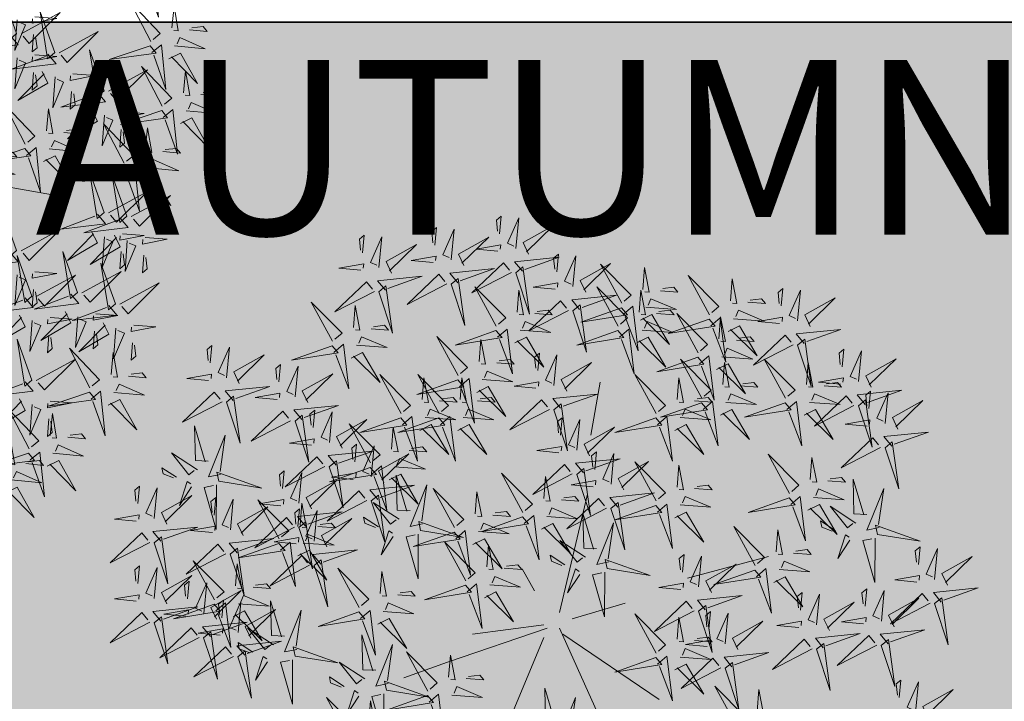
# Model space of a CAD drawing. Units: inches. Extents: x 1704 to 6393, y -157 to 1172.
# Tile 71 of 122: x 1920 to 1954, y 1010 to 1033. Entities that reach past the tile are written whole.
import ezdxf

# ---------------------------------------------------------------- set-up
doc = ezdxf.new("R2010")
doc.units = ezdxf.units.IN
doc.header["$MEASUREMENT"] = 0
for name, color, linetype, lineweight in [('A-ANNO-DIMS', 7, 'Continuous', 13), ('C-PROP', 7, 'Continuous', 35), ('L-shrub', 74, 'Continuous', 18), ('L-tree', 102, 'Continuous', 18)]:
    doc.layers.add(name, color=color, linetype=linetype, lineweight=lineweight)
doc.layers.add('L-HRDS-PATT', color=9, linetype='Continuous', lineweight=13, true_color=0xc5c1ba)
doc.styles.get("Standard").update_dxf_attribs({"font": 'arial.ttf'})
doc.dimstyles.get("Standard").update_dxf_attribs({"dimtxt": 6, "dimasz": 2, "dimexe": 0.18, "dimexo": 0.0625, "dimgap": 0.09, "dimtad": 0, "dimtih": 1, "dimtoh": 1, "dimdec": 1, "dimzin": 0, "dimdsep": 46, "dimlunit": 3, "dimtxsty": 'Standard', "dimblk": 'ARCHTICK', "dimcen": 0.09, "dimadec": 0, "dimazin": 0, "dimtfac": 1, "dimtdec": 1, "dimtofl": 0, "dimtmove": 0, "dimatfit": 3, "dimfxl": 1, "dimtolj": 1, "dimtzin": 0, "dimarcsym": 0})

# ---------------------------------------------------------------- blocks, each defined once
blk = doc.blocks.new('bamboo')
blk.add_line((390, 162.3), (546.4, 218.1))
at = {"layer": 'L-shrub'}
for p, q in [((43.5, 73), (278.2, 631.2)), ((-12.4, 39.5), (-247.1, 564.2)), ((-23.6, 61.9), (-370, 296.3)), ((32.3, 39.5), (390, 162.3)), ((43.5, 28.4), (300.5, 61.9)), ((-57.1, 6), (-247.1, -49.8)), ((-12.4, -16.3), (-113, -440.5)), ((77, -94.4), (121.7, -172.6)), ((-470.6, -139.1), (-761.2, -217.2)), ((-124.2, -652.6), (-157.7, -842.3))]:
    blk.add_line(p, q, dxfattribs=at)
for points in [[(-52.8, 429.4), (-9, 438.6), (-69, 289.1), (-50.5, 418.5)], [(455.6, 305.5), (421.7, 276.4), (402.2, 436.3), (448.3, 314)], [(617.5, 275.9), (618.2, 435.7), (661.3, 285.1), (628.5, 278.2)], [(747.2, 429.2), (823.6, 288.8), (713.3, 400), (738.7, 421.9)], [(672.1, 379.4), (666.1, 300.6), (649, 389), (664.8, 387.8)], [(-1334.9, 362.3), (-1315.1, 320.7), (-1424, 259.8), (-1327.8, 353.7)], [(-645.4, 388.3), (-569, 247.9), (-679.3, 359.1), (-653.9, 381)], [(-8.5, 381.7), (37.5, 380), (40.9, 255.2), (2.4, 384)], [(-1289.2, 342), (-1299.8, 231.9), (-1259.3, 323.3), (-1282.1, 333.4)], [(-720.5, 338.5), (-726.5, 259.7), (-743.5, 348.1), (-727.8, 346.9)], [(-606.2, 183.8), (-655.6, 331.4), (-632, 162.5), (-606.2, 183.8)], [(461.7, 281.3), (608.2, 333.7), (439.8, 306.7), (461.7, 281.3)], [(707.3, 283.4), (750.5, 349.5), (722.8, 263.8), (709.6, 272.4)], [(-1230.9, 288.8), (-1236.9, 225.9), (-1219.6, 240.1), (-1223.8, 280.1)], [(-363.6, 169.2), (-397.5, 140), (-417, 299.9), (-370.9, 177.6)], [(374.4, 279.9), (264.1, 288.2), (356.3, 249.6), (365.9, 272.6)], [(608.9, 262.7), (455.2, 287.4), (615.8, 229.9), (608.9, 262.7)], [(945.2, 153.2), (945.8, 313), (988.9, 162.4), (956.1, 155.5)], [(1141.3, 142.9), (1092, 290.5), (1115.5, 121.6), (1141.3, 142.9)], [(-1166, 102), (-1215.3, 249.6), (-1191.8, 80.7), (-1166, 102)], [(-933.9, 115.6), (-983.2, 263.3), (-959.7, 94.3), (-933.9, 115.6)], [(-590.5, 182.3), (-448.6, 255.9), (-562, 147.8), (-583.4, 173.7)], [(-425.4, 189.6), (-466.6, 169), (-529.7, 276.7), (-433.9, 182.4)], [(460.4, 265.6), (536.9, 125.2), (426.5, 236.4), (452, 258.3)], [(602.5, 238.5), (646.3, 247.7), (586.3, 98.2), (604.8, 227.6)], [(760.2, 248.9), (813.2, 214.4), (808.6, 236.2), (771.2, 251.2)], [(322.4, 220.5), (259.3, 225.2), (273.9, 208.3), (313.9, 213.2)], [(385.4, 215.7), (379.4, 137), (362.3, 225.4), (378.1, 224.2)], [(686, 221.8), (778.6, 161.5), (716.5, 239.7), (696.9, 224.1)], [(1035, 160.6), (1078.2, 226.8), (1050.5, 141.1), (1037.3, 149.7)], [(1157.1, 141.4), (1299, 214.9), (1185.5, 106.9), (1164.2, 132.8)], [(1264.2, 74.7), (1214.8, 222.3), (1238.4, 53.4), (1264.2, 74.7)], [(-918.2, 114.1), (-776.2, 187.7), (-889.7, 79.6), (-911, 105.5)], [(-630.5, 178.2), (-602.1, 143.7), (-762.3, 127.5), (-639.2, 171.1)], [(-357.5, 145), (-210.9, 197.3), (-379.3, 170.3), (-357.5, 145)], [(646.8, 190.8), (692.9, 189.1), (696.3, 64.3), (657.8, 193.1)], [(-1150.2, 100.5), (-1008.3, 174), (-1121.8, 66), (-1143.1, 91.9)], [(-444.7, 143.6), (-555, 151.8), (-462.9, 113.3), (-453.2, 136.3)], [(936.5, 139.9), (782.9, 164.7), (943.4, 107.2), (936.5, 139.9)], [(1279.9, 73.2), (1421.8, 146.8), (1308.4, 38.7), (1287, 64.6)], [(1441.7, 20.2), (1392.3, 167.8), (1415.9, -1.1), (1441.7, 20.2)], [(-958.2, 110.1), (-929.8, 75.6), (-1090, 59.3), (-966.8, 103)], [(-652.3, 116.9), (-632.5, 75.3), (-741.4, 14.4), (-645.2, 108.2)], [(-510.6, -20.7), (-560, 126.9), (-536.5, -42), (-510.6, -20.7)], [(-542.2, 106.2), (-463.6, 98.6), (-552.3, 83.4), (-550.8, 99.1)], [(-358.7, 129.2), (-282.3, -11.2), (-392.6, 100.1), (-367.2, 121.9)], [(639.5, 26), (598.3, 5.3), (535.3, 113), (631, 18.7)], [(701.3, 5.5), (667.4, -23.6), (647.9, 136.3), (694, 14)], [(930.2, 115.8), (973.9, 125), (914, -24.5), (932.5, 104.9)], [(1117, 137.3), (1145.4, 102.8), (985.2, 86.6), (1108.4, 130.2)], [(1013.6, 99.1), (1106.3, 38.8), (1044.2, 116.9), (1024.6, 101.4)], [(1087.9, 126.1), (1140.9, 91.6), (1136.3, 113.5), (1098.9, 128.4)], [(1220.1, -21.7), (1186.2, -50.9), (1166.7, 109), (1212.8, -13.3)], [(-1357.1, -48), (-1406.5, 99.6), (-1382.9, -69.3), (-1357.1, -48)], [(-1190.3, 96.4), (-1161.9, 61.9), (-1322.1, 45.7), (-1198.9, 89.3)], [(-606.6, 96.6), (-617.1, -13.5), (-576.7, 77.8), (-599.5, 88)], [(-496.8, 84.1), (-559.8, 88.8), (-545.3, 71.9), (-505.3, 76.8)], [(-433.8, 79.4), (-439.8, 0.6), (-456.8, 89), (-441.1, 87.9)], [(1095.3, 76), (1115.1, 34.4), (1006.1, -26.5), (1102.4, 67.3)], [(1158.3, -1.3), (1117.1, -21.9), (1054.1, 85.8), (1149.8, -8.5)], [(1457.4, 18.7), (1599.3, 92.2), (1485.9, -15.8), (1464.5, 10)], [(-979.9, 48.7), (-960.1, 7.1), (-1069.1, -53.8), (-972.8, 40.1)], [(-869.9, 38), (-791.3, 30.4), (-880, 15.2), (-878.5, 30.9)], [(-548.2, 43.3), (-554.2, -19.6), (-537, -5.4), (-541.1, 34.7)], [(-494.9, -22.2), (-353, 51.3), (-466.5, -56.7), (-487.8, -30.9)], [(319, -89.9), (285.1, -119.1), (265.6, 40.8), (311.8, -81.4)], [(974.5, 68.1), (1020.5, 66.3), (1023.9, -58.4), (985.4, 70.4)], [(1239.9, 69.2), (1268.3, 34.7), (1108.1, 18.4), (1231.3, 62.1)], [(1140.9, 55.7), (1130.4, -54.4), (1170.9, 36.9), (1148, 47)], [(1205.3, 65.3), (1283.9, 57.7), (1195.2, 42.5), (1196.7, 58.2)], [(-1341.4, -49.5), (-1199.5, 24), (-1312.9, -84), (-1334.3, -58.1)], [(-1212, 35.1), (-1192.2, -6.5), (-1301.2, -67.4), (-1204.9, 26.4)], [(-1166.4, 14.8), (-1176.9, -95.3), (-1136.4, -4), (-1159.3, 6.1)], [(-1102, 24.4), (-1023.4, 16.8), (-1112.1, 1.6), (-1110.6, 17.3)], [(-934.3, 28.4), (-944.8, -81.7), (-904.3, 9.6), (-927.2, 19.8)], [(257.2, -69.4), (216.1, -90.1), (153, 17.6), (248.8, -76.7)], [(707.4, -18.7), (854, 33.7), (685.6, 6.7), (707.4, -18.7)], [(1218.1, 7.8), (1238, -33.8), (1129, -94.7), (1225.2, -0.8)], [(1199.3, 2.4), (1193.3, -60.5), (1210.5, -46.3), (1206.4, -6.2)], [(1226.2, -46), (1372.8, 6.4), (1204.4, -20.6), (1226.2, -46)], [(1417.4, 14.6), (1445.8, -19.9), (1285.6, -36.1), (1408.7, 7.5)], [(-875.9, -24.9), (-881.9, -87.8), (-864.7, -73.6), (-868.8, -33.5)], [(-718.6, -144.5), (-752.5, -173.6), (-772, -13.7), (-725.8, -136)], [(-535, -26.3), (-506.5, -60.8), (-666.8, -77), (-543.6, -33.4)], [(-174.3, -160.5), (-173.7, -0.6), (-130.6, -151.3), (-163.4, -158.2)], [(620.2, -20.1), (509.9, -11.8), (602, -50.4), (611.7, -27.3)], [(706.2, -34.4), (782.6, -174.8), (672.3, -63.6), (697.7, -41.7)], [(1263.8, -12.5), (1253.3, -122.6), (1293.7, -31.3), (1270.9, -21.1)], [(1328.2, -2.9), (1406.8, -10.5), (1318.1, -25.7), (1319.6, -10)], [(-1381.4, -53.6), (-1353, -88.1), (-1513.2, -104.3), (-1390.1, -60.7)], [(-1108, -38.5), (-1114, -101.4), (-1096.8, -87.2), (-1100.9, -47.1)], [(-780.4, -124), (-821.5, -144.7), (-884.6, -37), (-788.8, -131.3)], [(325.1, -114.1), (471.7, -61.8), (303.3, -88.7), (325.1, -114.1)], [(868.3, -184.3), (818.9, -36.7), (842.4, -205.6), (868.3, -184.3)], [(1139, -47.3), (1028.7, -39.1), (1120.8, -77.6), (1130.5, -54.6)], [(1225, -61.7), (1301.4, -202.1), (1191.1, -90.8), (1216.5, -69)], [(1395.6, -46.8), (1415.5, -88.4), (1306.5, -149.2), (1402.7, -55.4)], [(1322.2, -65.8), (1316.2, -128.7), (1333.4, -114.5), (1329.3, -74.4)], [(1441.3, -67.1), (1430.8, -177.1), (1471.2, -85.8), (1448.4, -75.7)], [(1505.7, -57.4), (1584.3, -65), (1495.6, -80.2), (1497.1, -64.5)], [(-556.7, -87.7), (-536.9, -129.3), (-645.8, -190.1), (-549.6, -96.3)], [(-446.7, -98.3), (-368, -105.9), (-456.8, -121.2), (-455.3, -105.4)], [(-84.5, -153), (-41.3, -86.9), (-69, -172.5), (-82.2, -163.9)], [(568.1, -79.5), (505.1, -74.8), (519.6, -91.7), (559.6, -86.8)], [(631.1, -84.2), (625.1, -163), (608.1, -74.6), (623.8, -75.8)], [(1086.9, -106.8), (1023.9, -102.1), (1038.4, -119), (1078.4, -114.1)], [(1168.6, -225.3), (1119.3, -77.6), (1142.8, -246.6), (1168.6, -225.3)], [(1149.9, -111.5), (1143.9, -190.3), (1126.9, -101.9), (1142.6, -103)], [(-1403.2, -114.9), (-1383.3, -156.5), (-1492.3, -217.4), (-1396.1, -123.6)], [(-1357.5, -135.2), (-1368, -245.3), (-1327.6, -154), (-1350.4, -143.9)], [(-1293.1, -125.6), (-1214.5, -133.2), (-1303.2, -148.4), (-1301.7, -132.7)], [(-1143.7, -283.2), (-1143, -123.3), (-1099.9, -274), (-1132.7, -280.9)], [(-712.5, -168.7), (-565.9, -116.3), (-734.3, -143.3), (-712.5, -168.7)], [(-511, -108), (-521.6, -218), (-481.1, -126.7), (-503.9, -116.6)], [(237.9, -115.5), (127.6, -107.2), (219.7, -145.8), (229.4, -122.8)], [(323.9, -129.9), (400.4, -270.3), (290, -159), (315.4, -137.2)], [(494.6, -296.8), (495.3, -137), (538.4, -287.6), (505.6, -294.5)], [(926.2, -219.4), (885, -240.1), (822, -132.4), (917.7, -226.7)], [(884, -185.9), (1025.9, -112.3), (912.4, -220.4), (891.1, -194.5)], [(988, -239.9), (954.1, -269), (934.6, -109.2), (980.8, -231.4)], [(1441.7, -266.2), (1392.3, -118.6), (1415.9, -287.5), (1441.7, -266.2)], [(1499.7, -120.3), (1493.7, -183.2), (1510.9, -169), (1506.8, -128.9)], [(-799.7, -170.1), (-910, -161.8), (-817.9, -200.4), (-808.2, -177.3)], [(-452.7, -161.2), (-458.7, -224.1), (-441.4, -209.9), (-445.5, -169.8)], [(-183, -173.7), (-336.7, -149), (-176.1, -206.5), (-183, -173.7)], [(185.8, -175), (122.8, -170.2), (137.4, -187.2), (177.4, -182.3)], [(298.2, -260.3), (257, -281), (193.9, -173.3), (289.7, -267.6)], [(248.8, -179.7), (242.8, -258.4), (225.8, -170), (241.6, -171.2)], [(360, -280.8), (326.1, -310), (306.6, -150.1), (352.7, -272.3)], [(922.9, -320.7), (873.5, -173.1), (897.1, -342), (922.9, -320.7)], [(1184.4, -226.8), (1326.3, -153.2), (1212.8, -261.3), (1191.5, -235.4)], [(-1299.1, -188.5), (-1305.1, -251.4), (-1287.9, -237.2), (-1292, -197.1)], [(-1053.9, -275.7), (-1010.7, -209.6), (-1038.4, -295.3), (-1051.6, -286.6)], [(-713.7, -184.4), (-637.3, -324.8), (-747.6, -213.6), (-722.2, -191.7)], [(-189.3, -197.8), (-145.6, -188.6), (-205.5, -338.1), (-187, -208.8)], [(-105.9, -214.5), (-13.2, -274.9), (-75.4, -196.7), (-94.9, -212.2)], [(-31.6, -187.5), (21.3, -222), (16.7, -200.1), (-20.7, -185.2)], [(114.3, -335.4), (80.4, -364.5), (60.9, -204.6), (107, -326.9)], [(843.9, -189.9), (872.4, -224.4), (712.1, -240.6), (835.3, -197)], [(994.1, -264.1), (1140.7, -211.8), (972.3, -238.7), (994.1, -264.1)], [(1457.4, -267.7), (1599.3, -194.1), (1485.9, -302.2), (1464.5, -276.3)], [(-851.8, -229.5), (-914.8, -224.8), (-900.2, -241.7), (-860.3, -236.8)], [(-788.8, -234.2), (-794.8, -313), (-811.8, -224.6), (-796, -225.8)], [(-363.6, -376.3), (-397.5, -405.4), (-417, -245.5), (-370.9, -367.8)], [(-196.6, -388.9), (-246, -241.3), (-222.5, -410.2), (-196.6, -388.9)], [(-145, -245.6), (-99, -247.3), (-95.6, -372), (-134.1, -243.3)], [(52.5, -314.9), (11.3, -335.6), (-51.8, -227.9), (44, -322.2)], [(584.4, -289.3), (627.6, -223.2), (600, -308.9), (586.7, -300.3)], [(1144.3, -230.8), (1172.7, -265.3), (1012.5, -281.6), (1135.7, -237.9)], [(-1152.3, -296.4), (-1306, -271.7), (-1145.4, -329.2), (-1152.3, -296.4)], [(-841.4, -403.5), (-875.3, -432.7), (-894.8, -272.8), (-848.7, -395.1)], [(-425.4, -355.8), (-466.6, -376.5), (-529.7, -268.8), (-433.9, -363.1)], [(366.1, -305), (512.7, -252.7), (344.3, -279.6), (366.1, -305)], [(663.5, -416.2), (614.1, -268.5), (637.6, -437.5), (663.5, -416.2)], [(822.2, -251.3), (842, -292.9), (733.1, -353.8), (829.3, -259.9)], [(906.9, -265.5), (796.6, -257.2), (888.7, -295.8), (898.4, -272.8)], [(867.9, -271.6), (857.4, -381.7), (897.8, -290.4), (875, -280.2)], [(932.3, -262), (1010.9, -269.6), (922.2, -284.8), (923.7, -269.1)], [(938.6, -322.2), (1080.5, -248.7), (967.1, -356.7), (945.7, -330.8)], [(992.9, -279.9), (1069.3, -420.3), (959, -309), (984.4, -287.2)], [(1417.4, -271.7), (1445.8, -306.2), (1285.6, -322.5), (1408.7, -278.8)], [(-1158.7, -320.6), (-1114.9, -311.4), (-1174.8, -460.8), (-1156.4, -331.5)], [(-903.2, -383.1), (-944.4, -403.7), (-1007.5, -296), (-911.7, -390.3)], [(-1000.9, -310.2), (-948, -344.7), (-952.6, -322.9), (-990, -307.9)], [(-180.9, -390.4), (-39, -316.9), (-152.5, -424.9), (-173.8, -399)], [(120.3, -359.6), (266.9, -307.2), (98.5, -334.2), (120.3, -359.6)], [(278.8, -306.4), (168.6, -298.1), (260.7, -336.7), (270.4, -313.7)], [(486, -310), (332.3, -285.3), (492.9, -342.8), (486, -310)], [(1122.6, -292.2), (1142.4, -333.8), (1033.4, -394.7), (1129.7, -300.8)], [(1168.2, -312.5), (1157.7, -422.6), (1198.2, -331.3), (1175.3, -321.1)], [(1218.2, -474.1), (1218.9, -314.2), (1262, -464.9), (1229.2, -471.8)], [(1232.6, -302.9), (1311.2, -310.5), (1222.5, -325.7), (1224, -310)], [(-1075.2, -337.2), (-982.6, -397.6), (-1044.7, -319.4), (-1064.3, -334.9)], [(-357.5, -400.5), (-210.9, -348.1), (-379.3, -375.1), (-357.5, -400.5)], [(33.1, -361), (-77.2, -352.7), (14.9, -391.3), (24.6, -368.2)], [(364.9, -320.8), (441.3, -461.2), (331, -349.9), (356.4, -328.1)], [(479.7, -334.2), (523.4, -325), (463.5, -474.5), (482, -345.1)], [(563.1, -350.9), (655.8, -411.2), (593.6, -333), (574, -348.6)], [(637.4, -323.8), (690.3, -358.3), (685.7, -336.5), (648.3, -321.5)], [(679.2, -417.7), (821.1, -344.1), (707.7, -452.2), (686.3, -426.3)], [(898.6, -326.3), (927, -360.8), (766.8, -377), (889.9, -333.4)], [(854.8, -325), (791.8, -320.2), (806.4, -337.2), (846.3, -332.2)], [(917.8, -329.7), (911.8, -408.4), (894.8, -320), (910.5, -321.2)], [(926.3, -324.9), (920.3, -387.8), (937.5, -373.5), (933.4, -333.5)], [(1395.6, -333.1), (1415.5, -374.7), (1306.5, -435.6), (1402.7, -341.7)], [(1505.7, -343.8), (1584.3, -351.4), (1495.6, -366.6), (1497.1, -350.9)], [(-1114.4, -368.3), (-1068.3, -370), (-1064.9, -494.8), (-1103.4, -366)], [(-835.4, -427.8), (-688.8, -375.4), (-857.2, -402.4), (-835.4, -427.8)], [(-73.8, -511.6), (-123.1, -364), (-99.6, -532.9), (-73.8, -511.6)], [(119.1, -375.3), (195.6, -515.7), (85.2, -404.5), (110.7, -382.6)], [(226.8, -365.9), (163.8, -361.1), (178.3, -378.1), (218.3, -373.2)], [(289.8, -370.6), (283.8, -449.3), (266.8, -360.9), (282.5, -362.1)], [(524, -381.9), (570, -383.6), (573.4, -508.4), (534.9, -379.6)], [(660.4, -512.6), (626.5, -541.8), (607, -381.9), (653.1, -504.2)], [(876.8, -387.7), (896.6, -429.3), (787.7, -490.1), (883.9, -396.3)], [(1226.6, -365.8), (1220.6, -428.7), (1237.8, -414.5), (1233.7, -374.4)], [(1441.3, -353.4), (1430.8, -463.5), (1471.2, -372.2), (1448.4, -362)], [(-922.6, -429.1), (-1032.9, -420.9), (-940.7, -459.5), (-931.1, -436.4)], [(-444.7, -401.9), (-555, -393.6), (-462.9, -432.2), (-453.2, -409.1)], [(-358.7, -416.2), (-282.3, -556.6), (-392.6, -445.4), (-367.2, -423.5)], [(-221, -394.5), (-192.5, -429), (-352.8, -445.2), (-229.6, -401.6)], [(-19, -420.4), (-82, -415.7), (-67.4, -432.6), (-27.4, -427.7)], [(44, -425.1), (38, -503.9), (21, -415.5), (36.8, -416.7)], [(598.6, -492.1), (557.4, -512.8), (494.3, -405.1), (590.1, -499.4)], [(639.2, -421.7), (667.6, -456.2), (507.4, -472.5), (630.5, -428.8)], [(813.7, -538.9), (764.3, -391.3), (787.8, -560.2), (813.7, -538.9)], [(922.5, -407.9), (912, -518), (952.4, -426.7), (929.6, -416.6)], [(986.9, -398.3), (1065.5, -405.9), (976.8, -421.1), (978.3, -405.4)], [(1308, -466.6), (1351.2, -400.5), (1323.6, -486.2), (1310.3, -477.5)], [(1499.7, -406.7), (1493.7, -469.6), (1510.9, -455.4), (1506.8, -415.3)], [(-836.6, -443.5), (-760.1, -583.9), (-870.5, -472.6), (-845, -450.8)], [(-496.8, -461.3), (-559.8, -456.6), (-545.3, -473.5), (-505.3, -468.6)], [(-433.8, -466), (-439.8, -544.8), (-456.8, -456.4), (-441.1, -457.6)], [(-242.7, -455.8), (-222.9, -497.4), (-331.8, -558.3), (-235.6, -464.5)], [(-58, -513.1), (83.9, -439.6), (-29.6, -547.6), (-50.9, -521.7)], [(-1179.6, -607.1), (-1229, -459.4), (-1205.5, -628.4), (-1179.6, -607.1)], [(-974.6, -488.6), (-1037.7, -483.9), (-1023.1, -500.8), (-983.1, -495.9)], [(-911.6, -493.3), (-917.6, -572.1), (-934.7, -483.7), (-918.9, -484.8)], [(-197, -476.1), (-207.5, -586.2), (-167.1, -494.9), (-189.9, -484.8)], [(-132.6, -466.5), (-54, -474.1), (-142.8, -489.3), (-141.3, -473.6)], [(617.4, -483.1), (637.2, -524.7), (528.3, -585.6), (624.5, -491.7)], [(666.4, -536.8), (813, -484.5), (644.6, -511.4), (666.4, -536.8)], [(727.5, -493.8), (806.1, -501.4), (717.4, -516.6), (718.9, -500.9)], [(829.4, -540.4), (971.3, -466.8), (857.8, -574.9), (836.5, -549)], [(980.9, -461.2), (974.9, -524.1), (992.1, -509.9), (988, -469.8)], [(1209.6, -487.3), (1055.9, -462.6), (1216.5, -520.1), (1209.6, -487.3)], [(-98.1, -517.2), (-69.7, -551.7), (-229.9, -567.9), (-106.7, -524.3)], [(-138.6, -529.4), (-144.7, -592.3), (-127.4, -578.1), (-131.5, -538)], [(663.1, -503.4), (652.6, -613.5), (693, -522.2), (670.2, -512)], [(1203.3, -511.5), (1247, -502.3), (1187.1, -651.7), (1205.5, -522.4)], [(1286.7, -528.1), (1379.3, -588.5), (1317.2, -510.3), (1297.6, -525.8)], [(1361, -501.1), (1413.9, -535.6), (1409.3, -513.8), (1371.9, -498.8)], [(-1163.9, -608.6), (-1022, -535), (-1135.5, -643.1), (-1156.8, -617.2)], [(-363.6, -689.9), (-397.5, -719), (-417, -559.2), (-370.9, -681.4)], [(414.6, -689.9), (380.7, -719), (361.2, -559.2), (407.3, -681.4)], [(579.2, -538.2), (468.9, -529.9), (561.1, -568.5), (570.7, -545.5)], [(551.1, -689.9), (517.2, -719), (497.7, -559.2), (543.9, -681.4)], [(665.2, -552.6), (741.7, -693), (631.3, -581.7), (656.8, -559.9)], [(789.3, -544.5), (817.8, -578.9), (657.5, -595.2), (780.7, -551.6)], [(721.5, -556.7), (715.5, -619.6), (732.7, -605.4), (728.6, -565.3)], [(936.5, -702.5), (887.2, -554.9), (910.7, -723.8), (936.5, -702.5)], [(1247.5, -559.2), (1293.6, -560.9), (1297, -685.7), (1258.5, -556.9)], [(-425.4, -669.4), (-466.6, -690.1), (-529.7, -582.4), (-433.9, -676.7)], [(-119.8, -578.6), (-100, -620.2), (-209, -681), (-112.7, -587.2)], [(-74.2, -598.9), (-84.7, -708.9), (-44.2, -617.6), (-67, -607.5)], [(8.2, -743.4), (-41.2, -595.8), (-17.7, -764.7), (8.2, -743.4)], [(-9.8, -589.2), (68.8, -596.8), (-19.9, -612), (-18.4, -596.3)], [(352.8, -669.4), (311.6, -690.1), (248.5, -582.4), (344.3, -676.7)], [(489.3, -669.4), (448.2, -690.1), (385.1, -582.4), (480.9, -676.7)], [(527.1, -597.7), (464.1, -593), (478.7, -609.9), (518.7, -605)], [(590.2, -602.4), (584.1, -681.2), (567.1, -592.8), (582.9, -593.9)], [(-1204, -612.6), (-1175.5, -647.1), (-1335.8, -663.4), (-1212.6, -619.7)], [(-1084.1, -757), (-1133.4, -609.4), (-1109.9, -778.4), (-1084.1, -757)], [(-827.8, -744.4), (-861.7, -773.6), (-881.2, -613.7), (-835.1, -736)], [(-527.4, -744.4), (-561.3, -773.6), (-580.8, -613.7), (-534.7, -736)], [(767.6, -605.8), (787.4, -647.4), (678.5, -708.3), (774.7, -614.5)], [(813.3, -626.1), (802.7, -736.2), (843.2, -644.9), (820.4, -634.7)], [(877.7, -616.5), (956.3, -624.1), (867.5, -639.3), (869, -623.6)], [(952.3, -704), (1094.2, -630.5), (980.7, -738.5), (959.4, -712.7)], [(1182.3, -770.7), (1132.9, -623.1), (1156.5, -792), (1182.3, -770.7)], [(-889.6, -724), (-930.8, -744.6), (-993.8, -636.9), (-898.1, -731.2)], [(-589.2, -724), (-630.4, -744.6), (-693.5, -636.9), (-597.7, -731.2)], [(-357.5, -714.1), (-210.9, -661.7), (-379.3, -688.7), (-357.5, -714.1)], [(-15.8, -652.1), (-21.8, -715), (-4.6, -700.8), (-8.7, -660.7)], [(420.7, -714.1), (567.3, -661.7), (398.9, -688.7), (420.7, -714.1)], [(557.2, -714.1), (703.8, -661.7), (535.4, -688.7), (557.2, -714.1)], [(-1225.7, -674), (-1205.9, -715.6), (-1314.8, -776.5), (-1218.6, -682.6)], [(-1180, -694.3), (-1190.5, -804.4), (-1150.1, -713.1), (-1172.9, -702.9)], [(-1115.6, -684.7), (-1037, -692.3), (-1125.7, -707.5), (-1124.2, -691.8)], [(-1068.3, -758.6), (-926.4, -685), (-1039.9, -793.1), (-1061.2, -767.2)], [(23.9, -744.9), (165.8, -671.4), (52.3, -779.4), (31, -753.6)], [(346.4, -826.2), (312.4, -855.4), (293, -695.5), (339.1, -817.8)], [(871.6, -679.4), (865.6, -742.3), (882.9, -728.1), (878.8, -688)], [(1198, -772.2), (1339.9, -698.7), (1226.5, -806.7), (1205.1, -780.8)], [(-821.7, -768.6), (-675.1, -716.3), (-843.5, -743.3), (-821.7, -768.6)], [(-444.7, -715.5), (-555, -707.2), (-462.9, -745.8), (-453.2, -722.8)], [(-521.3, -768.6), (-374.8, -716.3), (-543.2, -743.3), (-521.3, -768.6)], [(-358.7, -729.9), (-282.3, -870.2), (-392.6, -759), (-367.2, -737.1)], [(284.5, -805.8), (243.4, -826.4), (180.3, -718.7), (276.1, -813.1)], [(333.5, -715.5), (223.2, -707.2), (315.3, -745.8), (325, -722.8)], [(470, -715.5), (359.7, -707.2), (451.8, -745.8), (461.5, -722.8)], [(419.5, -729.9), (495.9, -870.2), (385.6, -759), (411, -737.1)], [(556, -729.9), (632.4, -870.2), (522.1, -759), (547.5, -737.1)], [(912.2, -708.1), (940.6, -742.6), (780.4, -758.8), (903.6, -715.2)], [(-1108.4, -762.6), (-1079.9, -797.1), (-1240.2, -813.4), (-1117, -769.7)], [(-1121.6, -747.6), (-1127.7, -810.5), (-1110.4, -796.3), (-1114.5, -756.2)], [(-908.9, -770), (-1019.2, -761.8), (-927.1, -800.3), (-917.4, -777.3)], [(-608.6, -770), (-718.8, -761.8), (-626.7, -800.3), (-617.1, -777.3)], [(-496.8, -774.9), (-559.8, -770.2), (-545.3, -787.1), (-505.3, -782.2)], [(-433.8, -779.7), (-439.8, -858.4), (-456.8, -770), (-441.1, -771.2)], [(-16.2, -749), (12.3, -783.5), (-148, -799.7), (-24.8, -756.1)], [(281.4, -774.9), (218.4, -770.2), (232.9, -787.1), (272.9, -782.2)], [(344.4, -779.7), (338.4, -858.4), (321.4, -770), (337.1, -771.2)], [(417.9, -774.9), (354.9, -770.2), (369.5, -787.1), (409.4, -782.2)], [(480.9, -779.7), (474.9, -858.4), (457.9, -770), (473.7, -771.2)], [(890.5, -769.5), (910.3, -811.1), (801.3, -871.9), (897.6, -778.1)], [(1158, -776.3), (1186.4, -810.8), (1026.2, -827), (1149.3, -783.4)], [(-822.9, -784.4), (-746.5, -924.8), (-856.8, -813.5), (-831.4, -791.7)], [(-575.6, -887.6), (-616.8, -908.3), (-679.8, -800.6), (-584, -894.9)], [(-513.8, -908.1), (-547.7, -937.2), (-567.2, -777.3), (-521, -899.6)], [(-522.5, -784.4), (-446.1, -924.8), (-556.4, -813.5), (-531, -791.7)], [(-37.9, -810.4), (-18.1, -852), (-127, -912.8), (-30.8, -819)], [(352.4, -850.5), (499, -798.1), (330.6, -825.1), (352.4, -850.5)], [(936.1, -789.8), (925.6, -899.8), (966.1, -808.5), (943.2, -798.4)], [(1000.5, -780.1), (1079.1, -787.7), (990.4, -802.9), (991.9, -787.2)], [(-1130.1, -824), (-1110.3, -865.6), (-1219.3, -926.5), (-1123, -832.6)], [(-1084.5, -844.3), (-1095, -954.4), (-1054.5, -863.1), (-1077.3, -852.9)], [(-1020.1, -834.7), (-941.4, -842.3), (-1030.2, -857.5), (-1028.7, -841.8)], [(-961, -829.5), (-1024, -824.8), (-1009.5, -841.7), (-969.5, -836.8)], [(-898, -834.2), (-904, -913), (-921, -824.6), (-905.3, -825.7)], [(-865.6, -975.2), (-915, -827.6), (-891.5, -996.5), (-865.6, -975.2)], [(-660.6, -829.5), (-723.6, -824.8), (-709.1, -841.7), (-669.1, -836.8)], [(-597.6, -834.2), (-603.6, -913), (-620.7, -824.6), (-604.9, -825.7)], [(7.8, -830.7), (-2.8, -940.7), (37.7, -849.4), (14.9, -839.3)], [(72.2, -821), (150.8, -828.6), (62, -843.8), (63.5, -828.1)], [(265.2, -851.8), (154.9, -843.6), (247, -882.2), (256.7, -859.1)], [(735.1, -928.5), (693.9, -949.2), (630.8, -841.5), (726.6, -935.8)], [(796.9, -949), (763, -978.1), (743.5, -818.2), (789.6, -940.5)], [(994.5, -843), (988.5, -905.9), (1005.7, -891.7), (1001.6, -851.6)], [(1136.2, -837.6), (1156, -879.2), (1047.1, -940.1), (1143.3, -846.3)], [(-507.7, -932.3), (-361.1, -879.9), (-529.5, -906.9), (-507.7, -932.3)], [(-227.1, -1003.5), (-261, -1032.7), (-280.5, -872.8), (-234.3, -995)], [(209.8, -1003.5), (175.9, -1032.7), (156.4, -872.8), (202.6, -995)], [(351.2, -866.2), (427.7, -1006.6), (317.3, -895.4), (342.8, -873.5)], [(1181.9, -857.9), (1171.4, -968), (1211.8, -876.7), (1189, -866.6)], [(1246.3, -848.3), (1324.9, -855.9), (1236.2, -871.1), (1237.7, -855.4)], [(-1026.1, -897.6), (-1032.1, -960.5), (-1014.9, -946.3), (-1019, -906.2)], [(-849.9, -976.7), (-708, -903.2), (-821.4, -1011.2), (-842.8, -985.4)], [(-554.7, -1044.4), (-588.6, -1073.6), (-608.1, -913.7), (-562, -1036)], [(-288.9, -983), (-330, -1003.7), (-393.1, -896), (-297.3, -990.3)], [(148, -983), (106.8, -1003.7), (43.8, -896), (139.5, -990.3)], [(66.1, -883.9), (60.1, -946.8), (77.4, -932.6), (73.3, -892.5)], [(213.1, -911.3), (150.1, -906.6), (164.7, -923.5), (204.7, -918.6)], [(276.1, -916), (270.1, -994.8), (253.1, -906.4), (268.9, -907.6)], [(1240.3, -911.2), (1234.3, -974.1), (1251.5, -959.9), (1247.4, -919.8)], [(-616.5, -1023.9), (-657.7, -1044.6), (-720.8, -936.9), (-625, -1031.2)], [(-594.9, -933.7), (-705.2, -925.4), (-613.1, -964), (-603.4, -940.9)], [(-508.9, -948), (-432.5, -1088.4), (-542.8, -977.2), (-517.4, -955.3)], [(-60.1, -1097.9), (-109.5, -950.3), (-85.9, -1119.2), (-60.1, -1097.9)], [(803, -973.2), (949.5, -920.8), (781.1, -947.8), (803, -973.2)], [(-889.9, -980.8), (-861.5, -1015.3), (-1021.7, -1031.5), (-898.6, -987.9)], [(-647, -993.1), (-710, -988.4), (-695.4, -1005.3), (-655.5, -1000.4)], [(-584, -997.8), (-590, -1076.6), (-607, -988.2), (-591.3, -989.4)], [(-302.5, -1064.9), (-343.7, -1085.5), (-406.8, -977.8), (-311, -1072.1)], [(-240.7, -1085.3), (-274.6, -1114.5), (-294.1, -954.6), (-248, -1076.9)], [(-221, -1027.7), (-74.4, -975.4), (-242.8, -1002.3), (-221, -1027.7)], [(215.9, -1027.7), (362.5, -975.4), (194.1, -1002.3), (215.9, -1027.7)], [(715.7, -974.6), (605.5, -966.3), (697.6, -1004.9), (707.3, -981.8)], [(-548.6, -1068.6), (-402.1, -1016.3), (-570.5, -1043.2), (-548.6, -1068.6)], [(-308.2, -1029.1), (-418.5, -1020.8), (-326.4, -1059.4), (-316.7, -1036.4)], [(128.7, -1029.1), (18.4, -1020.8), (110.5, -1059.4), (120.2, -1036.4)], [(636.2, -1166.1), (586.8, -1018.5), (610.3, -1187.4), (636.2, -1166.1)], [(801.8, -988.9), (878.2, -1129.3), (767.9, -1018.1), (793.3, -996.2)], [(-911.7, -1042.2), (-891.9, -1083.8), (-1000.8, -1144.6), (-904.6, -1050.8)], [(-801.6, -1052.8), (-723, -1060.4), (-811.7, -1075.7), (-810.2, -1059.9)], [(-234.6, -1109.5), (-88.1, -1057.2), (-256.5, -1084.1), (-234.6, -1109.5)], [(-222.2, -1043.5), (-145.8, -1183.9), (-256.1, -1072.6), (-230.7, -1050.8)], [(-44.4, -1099.5), (97.5, -1025.9), (-15.9, -1134), (-37.3, -1108.1)], [(214.7, -1043.5), (291.1, -1183.9), (180.8, -1072.6), (206.2, -1050.8)], [(376.8, -1193.4), (327.4, -1045.8), (350.9, -1214.7), (376.8, -1193.4)], [(663.7, -1034), (600.7, -1029.3), (615.2, -1046.2), (655.2, -1041.3)], [(726.7, -1038.7), (720.7, -1117.5), (703.7, -1029.1), (719.4, -1030.3)], [(-866, -1062.5), (-876.5, -1172.5), (-836.1, -1081.2), (-858.9, -1071.1)], [(-635.9, -1070), (-746.1, -1061.7), (-654, -1100.3), (-644.4, -1077.3)], [(-549.8, -1084.4), (-473.4, -1224.8), (-583.8, -1113.5), (-558.3, -1091.7)], [(-360.3, -1088.6), (-423.3, -1083.8), (-408.7, -1100.8), (-368.8, -1095.8)], [(-297.3, -1093.3), (-303.3, -1172), (-320.3, -1083.6), (-304.5, -1084.8)], [(76.6, -1088.6), (13.6, -1083.8), (28.1, -1100.8), (68.1, -1095.8)], [(144.7, -1234.3), (95.3, -1086.7), (118.8, -1255.6), (144.7, -1234.3)], [(139.6, -1093.3), (133.6, -1172), (116.6, -1083.6), (132.3, -1084.8)], [(651.9, -1167.6), (793.8, -1094.1), (680.3, -1202.1), (659, -1176.3)], [(-807.6, -1115.7), (-813.6, -1178.6), (-796.4, -1164.4), (-800.5, -1124.4)], [(-687.9, -1129.5), (-751, -1124.7), (-736.4, -1141.7), (-696.4, -1136.8)], [(-624.9, -1134.2), (-630.9, -1213), (-648, -1124.6), (-632.2, -1125.7)], [(-321.9, -1110.9), (-432.1, -1102.7), (-340, -1141.2), (-330.3, -1118.2)], [(-235.8, -1125.3), (-159.4, -1265.7), (-269.7, -1154.4), (-244.3, -1132.6)], [(-84.4, -1103.5), (-56, -1138), (-216.2, -1154.2), (-93.1, -1110.6)], [(392.5, -1194.9), (534.4, -1121.4), (420.9, -1229.4), (399.6, -1203.5)], [(-106.2, -1164.9), (-86.3, -1206.5), (-195.3, -1267.4), (-99.1, -1173.5)], [(160.4, -1235.8), (302.3, -1162.3), (188.8, -1270.3), (167.5, -1244.4)], [(-373.9, -1170.4), (-436.9, -1165.7), (-422.4, -1182.6), (-382.4, -1177.7)], [(-310.9, -1175.1), (-316.9, -1253.9), (-334, -1165.5), (-318.2, -1166.6)], [(-60.5, -1185.2), (-71, -1295.3), (-30.6, -1204), (-53.4, -1193.8)], [(3.9, -1175.6), (82.5, -1183.2), (-6.2, -1198.4), (-4.7, -1182.7)], [(352.4, -1199), (380.9, -1233.5), (220.7, -1249.7), (343.8, -1206.1)], [(611.8, -1171.7), (640.3, -1206.2), (480.1, -1222.4), (603.2, -1178.8)], [(590.1, -1233.1), (609.9, -1274.7), (501, -1335.5), (597.2, -1241.7)], [(120.3, -1239.9), (148.8, -1274.4), (-11.4, -1290.6), (111.7, -1247)], [(-2.1, -1238.5), (-8.1, -1301.4), (9.1, -1287.1), (5, -1247.1)], [(330.7, -1260.4), (350.5, -1301.9), (241.6, -1362.8), (337.8, -1269)], [(440.8, -1271), (519.4, -1278.6), (430.7, -1293.8), (432.2, -1278.1)], [(635.8, -1253.4), (625.3, -1363.4), (665.7, -1272.1), (642.9, -1262)], [(700.2, -1243.7), (778.8, -1251.3), (690.1, -1266.6), (691.6, -1250.8)], [(98.6, -1301.3), (118.4, -1342.9), (9.5, -1403.7), (105.7, -1309.9)], [(376.4, -1280.6), (365.9, -1390.7), (406.3, -1299.4), (383.5, -1289.3)], [(144.3, -1321.5), (133.8, -1431.6), (174.2, -1340.3), (151.4, -1330.2)], [(208.7, -1311.9), (287.3, -1319.5), (198.6, -1334.7), (200.1, -1319)], [(434.8, -1333.9), (428.8, -1396.8), (446, -1382.6), (441.9, -1342.5)], [(694.2, -1306.6), (688.2, -1369.5), (705.4, -1355.3), (701.3, -1315.3)], [(202.7, -1374.8), (196.7, -1437.7), (213.9, -1423.5), (209.8, -1383.4)]]:
    blk.add_lwpolyline(points, dxfattribs=at)
blk = doc.blocks.new('_ArchTick')
at = {"color": 0, "linetype": 'ByBlock', "const_width": 0.15}
blk.add_lwpolyline([(-0.5, -0.5), (0.5, 0.5)], dxfattribs=at)
blk = doc.blocks.new('*D80')
at = {"layer": 'A-ANNO-DIMS', "color": 0, "lineweight": -2, "transparency": 16777216}
for p, q in [((2018.966, 1025.001), (2018.966, 1029.096)), ((2045.487, 1025.001), (2045.487, 1029.096)), ((2018.966, 1028.916), (2016.966, 1028.916)), ((2045.487, 1028.916), (2018.966, 1028.916))]:
    blk.add_line(p, q, dxfattribs=at)
at = {"layer": 'Defpoints', "color": 0, "lineweight": -3, "transparency": 16777216}
for p in [(2018.966, 1028.916), (2018.966, 1024.938), (2045.487, 1024.938)]:
    blk.add_point(p, dxfattribs=at)
at = {"layer": 'A-ANNO-DIMS', "color": 0, "lineweight": -2, "transparency": 16777216, "xscale": 2, "yscale": 2, "zscale": 2, "rotation": 180}
blk.add_blockref('_ArchTick', (2018.966, 1028.916), dxfattribs=at)
at = {"layer": 'A-ANNO-DIMS', "color": 0, "lineweight": -2, "transparency": 16777216, "xscale": 2, "yscale": 2, "zscale": 2}
blk.add_blockref('_ArchTick', (2045.487, 1028.916), dxfattribs=at)
at = {"layer": 'A-ANNO-DIMS', "color": 0, "transparency": 16777216, "insert": (1967.173, 1028.916), "char_height": 6, "attachment_point": 5}
blk.add_mtext('\\A1;AUTUMN SHRUB 27 TYP.', dxfattribs=at)
blk = doc.blocks.new('*D94')
at = {"layer": 'A-ANNO-DIMS', "color": 0, "lineweight": -2, "transparency": 16777216}
for p, q in [((1898.349, 895.275), (1898.349, 1105.287)), ((2073.349, 895.275), (2073.349, 1105.287)), ((1898.349, 1105.107), (1979.39, 1105.107)), ((2073.349, 1105.107), (1992.307, 1105.107))]:
    blk.add_line(p, q, dxfattribs=at)
at = {"layer": 'Defpoints', "color": 0, "lineweight": -3, "transparency": 16777216}
for p in [(2073.349, 1105.107), (1898.349, 895.213), (2073.349, 895.213)]:
    blk.add_point(p, dxfattribs=at)
at = {"layer": 'A-ANNO-DIMS', "color": 0, "lineweight": -2, "transparency": 16777216, "xscale": 2, "yscale": 2, "zscale": 2, "rotation": 180}
blk.add_blockref('_ArchTick', (1898.349, 1105.107), dxfattribs=at)
at = {"layer": 'A-ANNO-DIMS', "color": 0, "lineweight": -2, "transparency": 16777216, "xscale": 2, "yscale": 2, "zscale": 2}
blk.add_blockref('_ArchTick', (2073.349, 1105.107), dxfattribs=at)
at = {"layer": 'A-ANNO-DIMS', "color": 0, "transparency": 16777216, "insert": (1985.849, 1105.107), "char_height": 6, "attachment_point": 5}
blk.add_mtext('\\A1;175', dxfattribs=at)

msp = doc.modelspace()

# ---------------------------------------------------------------- hatches: boundary and pattern name
at = {"layer": 'L-HRDS-PATT', "transparency": 33554643}
h = msp.add_hatch(color=256, dxfattribs=at)
h.dxf.hatch_style = 1
h.paths.add_polyline_path([(2065.589, 1033.213), (1898.349, 1033.213), (1898.349, 895.213), (2065.589, 895.213)])

# ---------------------------------------------------------------- linework, layer by layer
at = {"layer": 'C-PROP'}
msp.add_line((2723.349, 1033.213), (1898.349, 1033.213), dxfattribs=at)

# ---------------------------------------------------------------- block references
at = {"layer": 'L-tree', "xscale": 0.0095734028514679, "yscale": 0.0095734028514679, "zscale": 0.0095734028514679}
for p, rotation in [((1913.269, 1028.796), 89.99999999999996), ((1938.628, 1012.792), 180)]:
    msp.add_blockref('bamboo', p, dxfattribs=dict(at, rotation=rotation))

# ---------------------------------------------------------------- dimensions: what is measured, and where the dimension line sits
at = {"layer": 'A-ANNO-DIMS'}
dim = msp.add_linear_dim(base=(2073.349, 1105.107), p1=(1898.349, 895.213), p2=(2073.349, 895.213), dimstyle='Standard', override={"dimdec": 0, "dimlfac": 1, "dimrnd": 0, "dimzin": 0, "dimdsep": 46, "dimlunit": 2}, dxfattribs=at)
dim.commit()
dim.dimension.update_dxf_attribs({"geometry": '*D94', "text_midpoint": (1985.849, 1105.107)})
dim = msp.add_linear_dim(base=(2018.966, 1028.916), p1=(2045.487, 1024.938), p2=(2018.966, 1024.938), angle=180, text='AUTUMN SHRUB <> TYP.', dimstyle='Standard', override={"dimdec": 0, "dimlfac": 1, "dimrnd": 0, "dimzin": 0, "dimdsep": 46, "dimlunit": 2}, dxfattribs=at)
dim.commit()
dim.dimension.update_dxf_attribs({"geometry": '*D80', "text_midpoint": (1967.173, 1028.916)})

doc.saveas('drawing.dxf')
